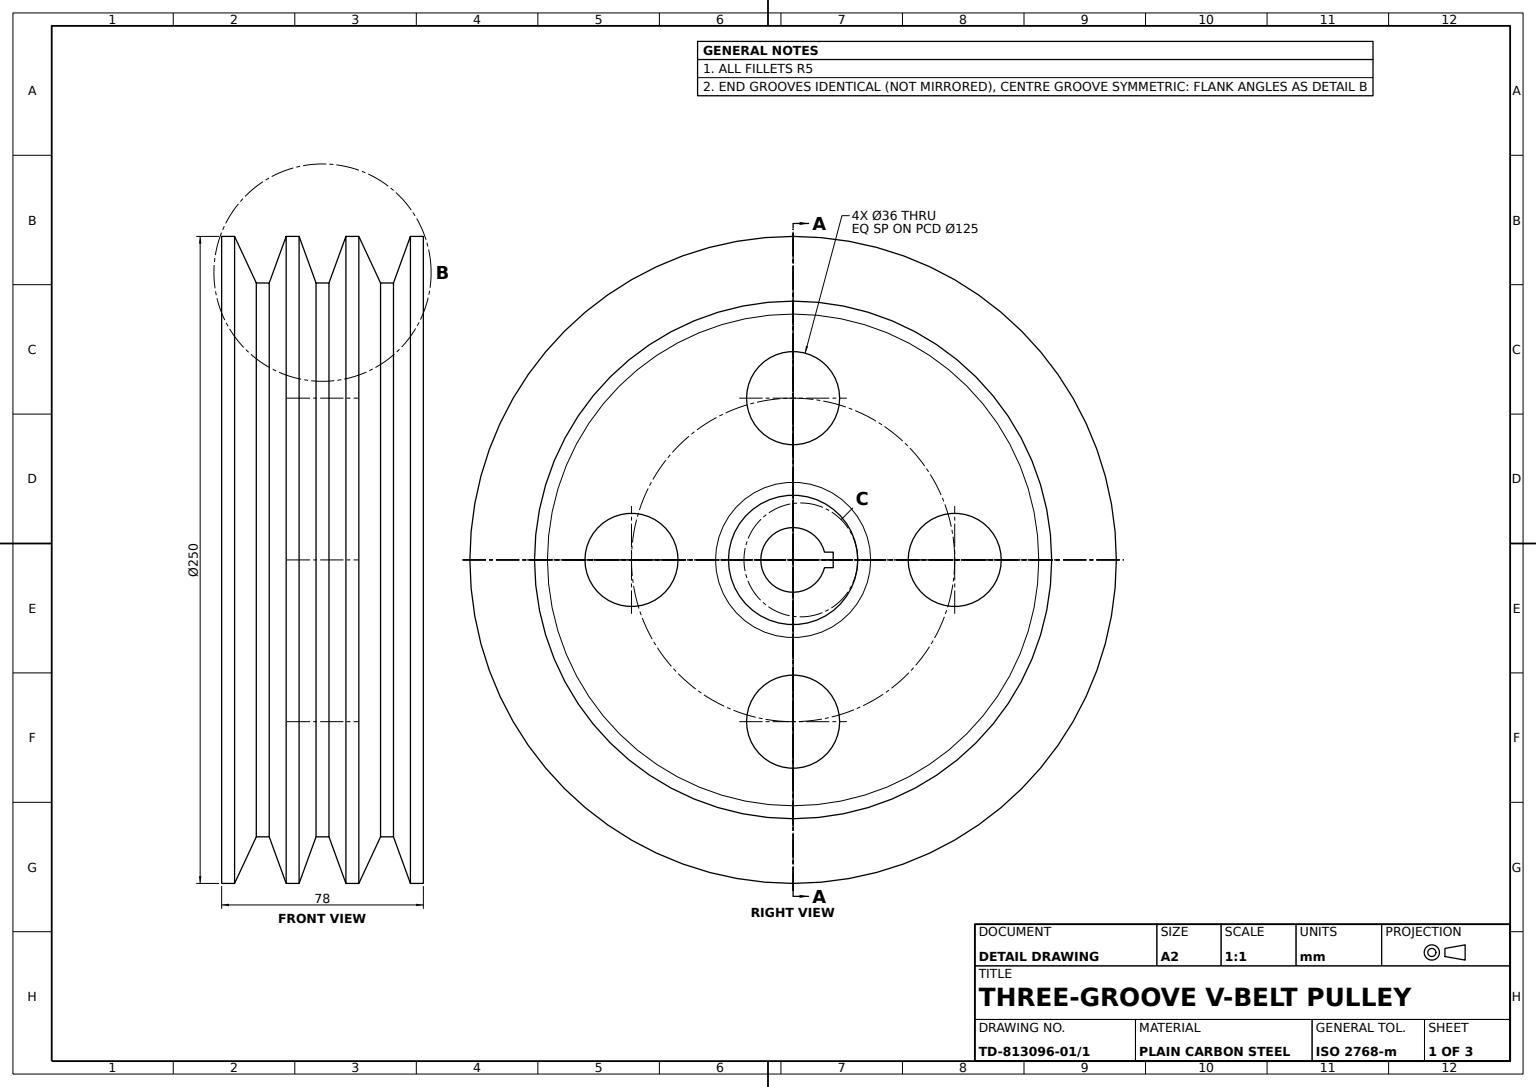
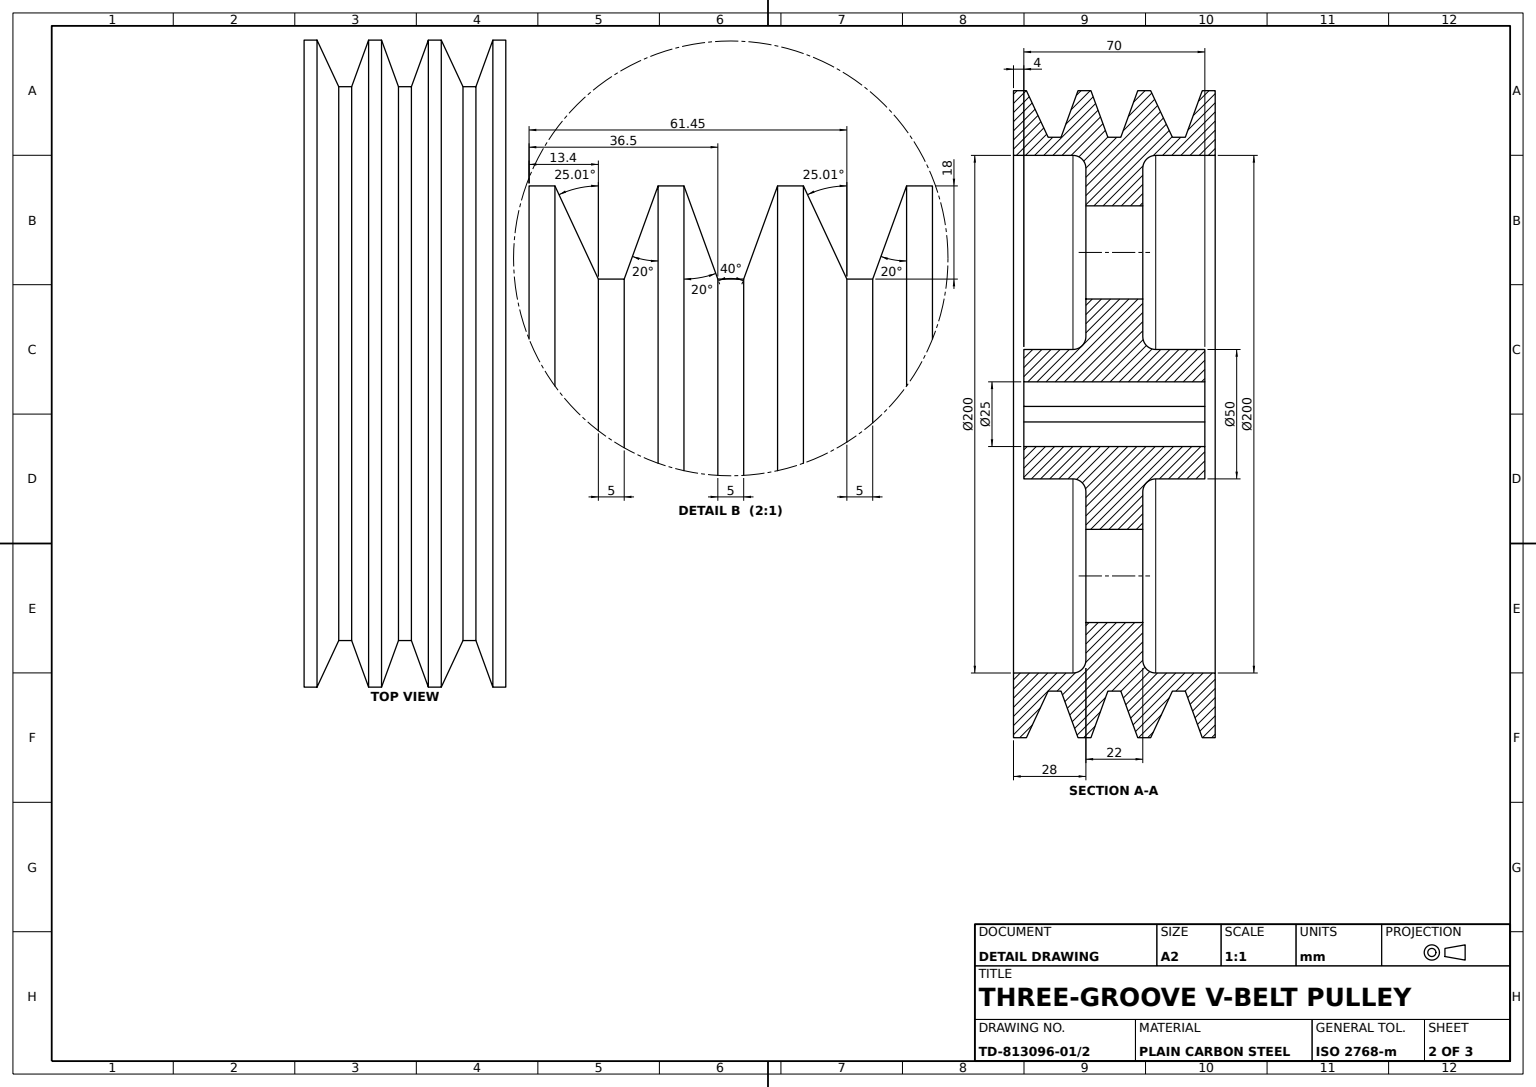
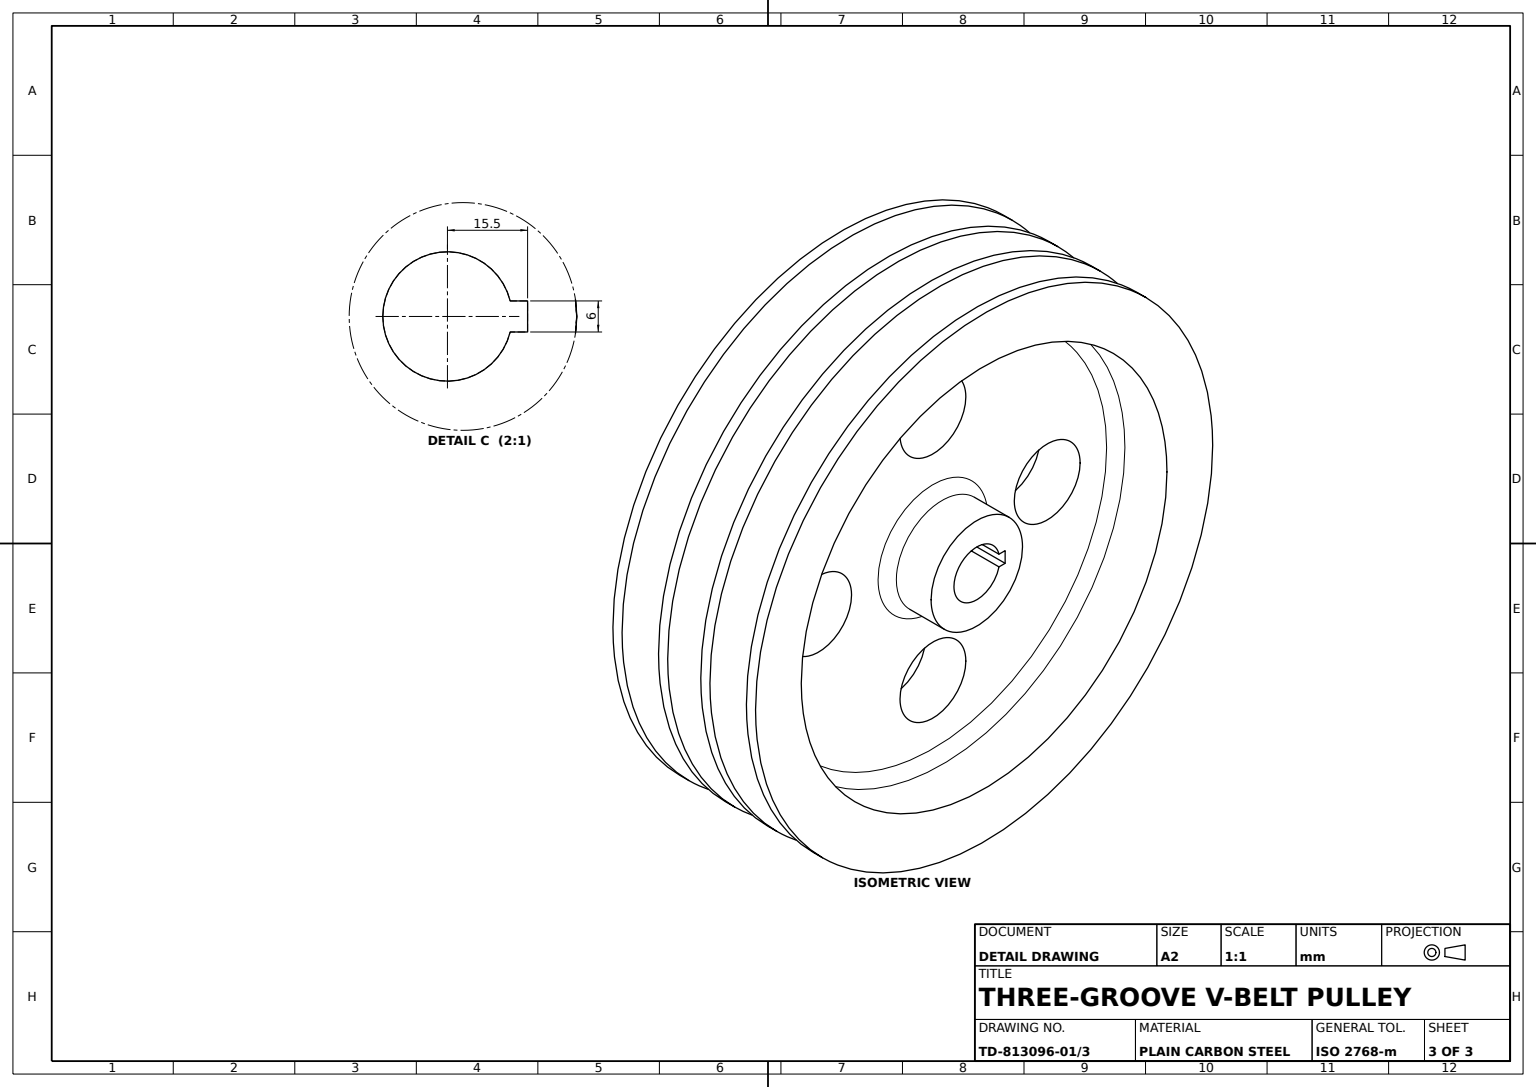
SolidWorks part; units mm, degrees
material "Plain Carbon Steel"
ref_plane "Front Plane" through (0, 0, 0) normal (0, 0, 1) x (1, 0, 0)
ref_plane "Top Plane" through (0, 0, 0) normal (0, 1, 0) x (1, 0, 0)
ref_plane "Right Plane" through (0, 0, 0) normal (1, 0, 0) x (0, 0, -1)
sketch "Pulley Profile Sketch" plane through (0, 0, 0) normal (0, 0, 1) x (1, 0, 0)
  line L0 (-35, 12.5) -> (35, 12.5)
  line L1 (35, 12.5) -> (35, 25)
  line L2 (35, 25) -> (11, 25)
  line L3 (11, 25) -> (11, 100)
  line L4 (11, 100) -> (39, 100)
  line L5 (39, 100) -> (39, 125)
  line L6 (39, 125) -> (34, 125)
  line L7 (34, 125) -> (27.4485, 107)
  line L8 (27.4485, 107) -> (22.4485, 107)
  line L9 (22.4485, 107) -> (14.0515, 125)
  line L10 (14.0515, 125) -> (9.0515, 125)
  line L11 (9.0515, 125) -> (2.5, 107)
  line L12 (2.5, 107) -> (-2.5, 107)
  line L13 (-2.5, 107) -> (-9.0515, 125)
  line L14 (-9.0515, 125) -> (-14.0515, 125)
  line L15 (-14.0515, 125) -> (-20.6029, 107)
  line L16 (-20.6029, 107) -> (-25.6029, 107)
  line L17 (-25.6029, 107) -> (-34, 125)
  line L18 (-34, 125) -> (-39, 125)
  line L19 (-39, 125) -> (-39, 100)
  line L20 (-39, 100) -> (-11, 100)
  line L21 (-11, 100) -> (-11, 25)
  line L22 (-11, 25) -> (-35, 25)
  line L23 (-35, 25) -> (-35, 12.5)
  line L24 (0, 0) -> (0, 305.5851) construction
  line L25 (-52.0758, 0) -> (67.7786, 0) construction
  dimension "D1" = 12.5
  dimension "D2" = 25
  dimension "D3" = 70
  dimension "D4" = 22
  dimension "D5" = 40
  dimension "D6" = 5
  dimension "D7" = 5
  dimension "D8" = 5
  dimension "D9" = 5
  dimension "D10" = 5
  dimension "D11" = 5
  dimension "D12" = 5
  dimension "D13" = 18
  dimension "D14" = 25
  dimension "D15" = 78
  dimension "D16" = 125
revolve "Pulley Body Revolve" add sketch "Pulley Profile Sketch" angle 360 about L25
fillet "Edge Fillet R5 A" radius 5 1 edges at (11, 0, 100)
fillet "Edge Fillet R5 B" radius 5 1 edges at (11, 0, 25)
fillet "Edge Fillet R5 C" radius 5 2 edges at (-11, 0, 100) (-11, 0, 25)
sketch "Keyway Sketch" plane through (35, 0, 0) normal (1, 0, 0) x (0, 0, -1)
  line L5 (12.1347, 3) -> (15.5, 3)
  line L7 (12.1347, -3) -> (15.5, -3)
  line L8 (15.5, 3) -> (15.5, -3)
  line L9 (9.5, 3) -> (15.5, -3) construction
  line L10 (9.5, -3) -> (15.5, 3) construction
  circle A0 centre (0, 0) radius 12.5 construction
  arc A1 (12.1347, -3) -> (12.1347, 3) centre (0, 0) ccw
  point P0 (12.5, 0)
  dimension "D1" = 6
  dimension "D2" = 6
extrude "Keyway 6x6" cut sketch "Keyway Sketch" against normal blind 80
sketch "Lightening Holes Sketch" plane through (11, 0, 0) normal (1, 0, 0) x (0, 0, -1)
  circle A0 centre (0, 0) radius 62.5 construction
  circle A1 centre (0, 62.5) radius 18
  circle A2 centre (62.5, 0) radius 18
  circle A3 centre (0, -62.5) radius 18
  circle A4 centre (-62.5, 0) radius 18
  point P14 (0, 0)
  dimension "D1" = 125
  dimension "D2" = 36
  dimension "D3" = 4
extrude "Lightening Holes 4xØ36" cut sketch "Lightening Holes Sketch" against normal mid plane 90
